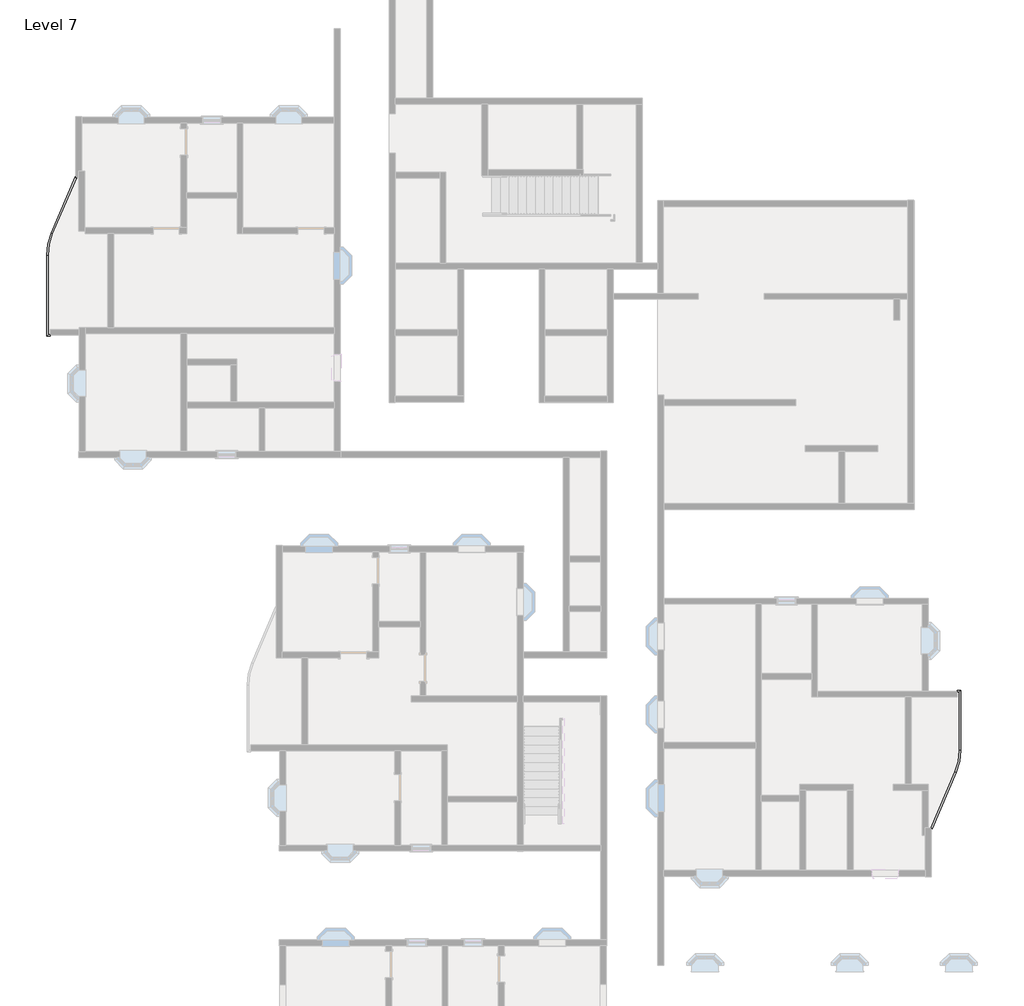
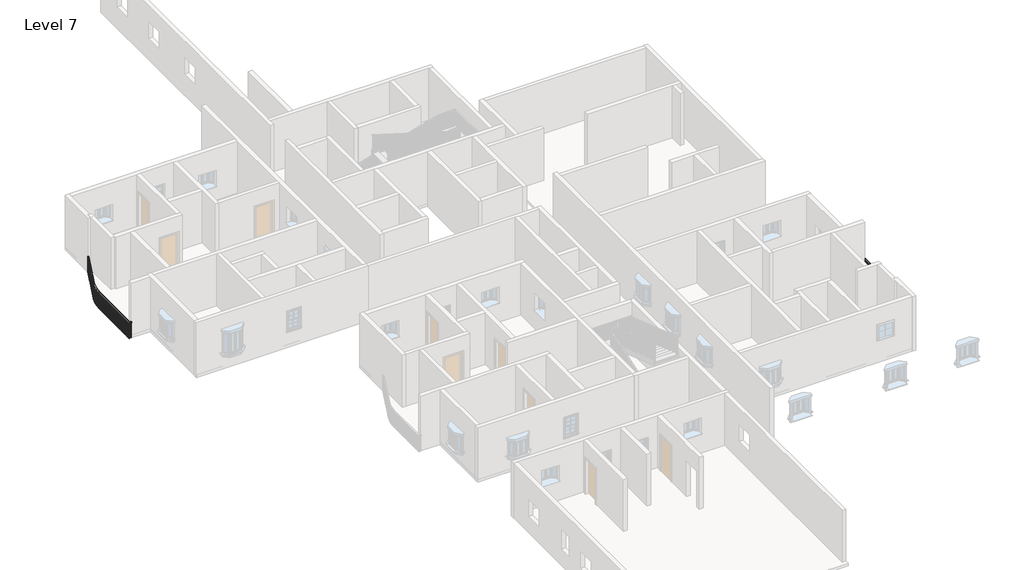
# One storey, part 9 of 14: 2 railings.
"""IFC4 building model written with IfcOpenShell, lengths in millimetres."""

from ifc_helpers import new_model, si_unit, frame, origin, place, context, project, spatial, polyline, circle_curve, outline, extrude, element, save
from ifc_brep_helpers import plane_surface, cylinder_surface, revolved_surface, advanced_brep

model = new_model("IFC4")

# Units and contexts
model_context = context("Model", 3, world=origin())
ifc_project = project(units=[si_unit("LENGTHUNIT", "METRE", prefix="MILLI")], contexts=[model_context])

# Site, building, storey
site = spatial("IfcSite", under=ifc_project)
building = spatial("IfcBuilding", under=site)
storey = spatial("IfcBuildingStorey", under=building, Name="Level 7", Elevation=18288.0)

# Railings
placement = place(None, origin())
element("IfcRailing", 1, ObjectType="Handrail - Rectangular", at=placement, inside=storey, context=model_context, shape_type="SolidModel", body=[
    advanced_brep(
    [(-19327.739878, 12446.0257339, 19202.4), (-19327.739878, 12446.0257339, 19151.6), (-19374.4383922, 12466.022953, 19151.6), (-19374.4383922, 12466.022953, 19202.4), (-20162.483418, 10496.6905323, 19202.4), (-20162.483418, 10496.6905323, 19151.6), (-20209.1819322, 10516.6877514, 19151.6), (-20209.1819322, 10516.6877514, 19202.4), (-20316.2891351, 9746.7948172, 19151.6), (-20316.2891351, 9746.7948172, 19202.4), (-20367.0891351, 9746.7948172, 19151.6), (-20367.0891351, 9746.7948172, 19202.4), (-20316.2891351, 7005.2583494, 19202.4), (-20316.2891351, 7005.2583494, 19151.6), (-20367.0891351, 6954.4583494, 19151.6), (-20367.0891351, 6954.4583494, 19202.4), (-20240.0891351, 7005.2583494, 19202.4), (-20240.0891351, 6954.4583494, 19202.4), (-20240.0891351, 6954.4583494, 19151.6), (-20240.0891351, 7005.2583494, 19151.6)],
    [
        (0, 1),
        (1, 2),
        (2, 3),
        (3, 0),
        (0, 4),
        (4, 5),
        (5, 1),
        (5, 6),
        (6, 2),
        (6, 7),
        (7, 3),
        (7, 4),
        (8, 5, circle_curve(frame((-18411.2891351, 9746.7948172, 19151.6), z_axis=(0.0, 0.0, -1.0), x_axis=(-0.919262090762392, 0.3936460446735823, 0.0)), 1905.0)),
        (4, 9, circle_curve(frame((-18411.2891351, 9746.7948172, 19202.4), z_axis=(0.0, 0.0, 1.0), x_axis=(-0.919262090762392, 0.3936460446735823, 0.0)), 1905.0)),
        (9, 8),
        (10, 6, circle_curve(frame((-18411.2891351, 9746.7948172, 19151.6), z_axis=(0.0, 0.0, -1.0), x_axis=(-0.919262090762392, 0.3936460446735823, 0.0)), 1955.8)),
        (8, 10),
        (11, 7, circle_curve(frame((-18411.2891351, 9746.7948172, 19202.4), z_axis=(0.0, 0.0, -1.0), x_axis=(-0.919262090762392, 0.3936460446735823, 0.0)), 1955.8)),
        (10, 11),
        (11, 9),
        (9, 12),
        (12, 13),
        (13, 8),
        (13, 14),
        (14, 10),
        (14, 15),
        (15, 11),
        (15, 12),
        (16, 17),
        (17, 18),
        (18, 19),
        (19, 16),
        (12, 16),
        (19, 13),
        (18, 14),
        (17, 15),
    ],
    [
        plane_surface(frame((-19351.0891351, 12456.0243434, 19202.4), z_axis=(0.3936460446735829, 0.9192620907623917, 0.0), x_axis=(0.9192620907623917, -0.3936460446735829, 0.0))),
        plane_surface(frame((-19327.739878, 12446.0257339, 19202.4), z_axis=(0.9192620907623915, -0.3936460446735834, 0.0), x_axis=(-0.3936460446735834, -0.9192620907623915, 0.0))),
        plane_surface(frame((-19327.739878, 12446.0257339, 19151.6), z_axis=(0.0, 0.0, -1.0000000000000002), x_axis=(-0.3936460446735834, -0.9192620907623915, 0.0))),
        plane_surface(frame((-19374.4383922, 12466.022953, 19151.6), z_axis=(-0.9192620907623916, 0.393646044673583, 0.0), x_axis=(-0.393646044673583, -0.9192620907623916, 0.0))),
        plane_surface(frame((-19374.4383922, 12466.022953, 19202.4), z_axis=(0.0, 0.0, 1.0), x_axis=(-0.393646044673583, -0.9192620907623916, 0.0))),
        revolved_surface(polyline([(-20162.483418002357, 10496.690532303173, 19202.4), (-20162.483418002357, 10496.690532303173, 19151.6)]), (-18411.2891351, 9746.7948172, 19202.4), (0.0, 0.0, 1.0)),
        plane_surface(frame((-18411.2891351, 9746.7948172, 19151.6), z_axis=(0.0, 0.0, -1.0), x_axis=(-0.919262090762392, 0.3936460446735823, 0.0))),
        cylinder_surface(frame((-18411.2891351, 9746.7948172, 19202.4), z_axis=(0.0, 0.0, 1.0), x_axis=(-0.919262090762392, 0.3936460446735823, 0.0)), 1955.8),
        plane_surface(frame((-18411.2891351, 9746.7948172, 19202.4), z_axis=(0.0, 0.0, 1.0), x_axis=(-0.919262090762392, 0.3936460446735823, 0.0))),
        plane_surface(frame((-20316.2891351, 9746.7948172, 19202.4), z_axis=(1.0, 0.0, 0.0), x_axis=(0.0, -1.0, 0.0))),
        plane_surface(frame((-20316.2891351, 9746.7948172, 19151.6), z_axis=(0.0, 0.0, -1.0), x_axis=(0.0, -1.0, 0.0))),
        plane_surface(frame((-20367.0891351, 9746.7948172, 19151.6), z_axis=(-1.0, 0.0, 0.0), x_axis=(0.0, -1.0, 0.0))),
        plane_surface(frame((-20367.0891351, 9746.7948172, 19202.4), z_axis=(0.0, 0.0, 1.0), x_axis=(0.0, -1.0, 0.0))),
        plane_surface(frame((-20240.0891351, 6979.8583494, 19202.4), z_axis=(1.0, 0.0, 0.0), x_axis=(0.0, 1.0, 0.0))),
        plane_surface(frame((-20316.2891351, 7005.2583494, 19202.4), z_axis=(0.0, 1.0, 0.0), x_axis=(1.0, 0.0, 0.0))),
        plane_surface(frame((-20316.2891351, 7005.2583494, 19151.6), z_axis=(0.0, 0.0, -1.0), x_axis=(1.0, 0.0, 0.0))),
        plane_surface(frame((-20367.0891351, 6954.4583494, 19151.6), z_axis=(0.0, -1.0, 0.0), x_axis=(1.0, 0.0, 0.0))),
        plane_surface(frame((-20367.0891351, 6954.4583494, 19202.4), z_axis=(0.0, 0.0, 1.0), x_axis=(1.0, 0.0, 0.0))),
    ],
    [
        (0, [[1, 2, 3, 4]]),
        (1, [[-1, 5, 6, 7]]),
        (2, [[-2, -7, 8, 9]]),
        (3, [[-3, -9, 10, 11]]),
        (4, [[-4, -11, 12, -5]]),
        (5, [[13, -6, 14, 15]]),
        (6, [[16, -8, -13, 17]]),
        (7, [[18, -10, -16, 19]]),
        (8, [[-14, -12, -18, 20]]),
        (9, [[-15, 21, 22, 23]]),
        (10, [[-17, -23, 24, 25]]),
        (11, [[-19, -25, 26, 27]]),
        (12, [[-20, -27, 28, -21]]),
        (13, [[29, 30, 31, 32]]),
        (14, [[-22, 33, -32, 34]]),
        (15, [[-24, -34, -31, 35]]),
        (16, [[-26, -35, -30, 36]]),
        (17, [[-28, -36, -29, -33]]),
    ],
),
    extrude(outline(polyline([(-20351.2141351, 7013.1198172), (-20332.1641351, 7013.1198172), (-20332.1641351, 6994.0698172), (-20351.2141351, 6994.0698172), (-20351.2141351, 7013.1198172)])), frame((0.0, 0.0, 18288.0), z_axis=(0.0, 0.0, 1.0), x_axis=(1.0, 0.0, 0.0)), (0.0, 0.0, 1.0), 863.6),
    extrude(outline(polyline([(-20351.2141351, 7114.7198172), (-20332.1641351, 7114.7198172), (-20332.1641351, 7095.6698172), (-20351.2141351, 7095.6698172), (-20351.2141351, 7114.7198172)])), frame((0.0, 0.0, 18288.0), z_axis=(0.0, 0.0, 1.0), x_axis=(1.0, 0.0, 0.0)), (0.0, 0.0, 1.0), 863.6),
    extrude(outline(polyline([(-20351.2141351, 7216.3198172), (-20332.1641351, 7216.3198172), (-20332.1641351, 7197.2698172), (-20351.2141351, 7197.2698172), (-20351.2141351, 7216.3198172)])), frame((0.0, 0.0, 18288.0), z_axis=(0.0, 0.0, 1.0), x_axis=(1.0, 0.0, 0.0)), (0.0, 0.0, 1.0), 863.6),
    extrude(outline(polyline([(-20351.2141351, 7317.9198172), (-20332.1641351, 7317.9198172), (-20332.1641351, 7298.8698172), (-20351.2141351, 7298.8698172), (-20351.2141351, 7317.9198172)])), frame((0.0, 0.0, 18288.0), z_axis=(0.0, 0.0, 1.0), x_axis=(1.0, 0.0, 0.0)), (0.0, 0.0, 1.0), 863.6),
    extrude(outline(polyline([(-20351.2141351, 7419.5198172), (-20332.1641351, 7419.5198172), (-20332.1641351, 7400.4698172), (-20351.2141351, 7400.4698172), (-20351.2141351, 7419.5198172)])), frame((0.0, 0.0, 18288.0), z_axis=(0.0, 0.0, 1.0), x_axis=(1.0, 0.0, 0.0)), (0.0, 0.0, 1.0), 863.6),
    extrude(outline(polyline([(-20351.2141351, 7521.1198172), (-20332.1641351, 7521.1198172), (-20332.1641351, 7502.0698172), (-20351.2141351, 7502.0698172), (-20351.2141351, 7521.1198172)])), frame((0.0, 0.0, 18288.0), z_axis=(0.0, 0.0, 1.0), x_axis=(1.0, 0.0, 0.0)), (0.0, 0.0, 1.0), 863.6),
    extrude(outline(polyline([(-20351.2141351, 7622.7198172), (-20332.1641351, 7622.7198172), (-20332.1641351, 7603.6698172), (-20351.2141351, 7603.6698172), (-20351.2141351, 7622.7198172)])), frame((0.0, 0.0, 18288.0), z_axis=(0.0, 0.0, 1.0), x_axis=(1.0, 0.0, 0.0)), (0.0, 0.0, 1.0), 863.6),
    extrude(outline(polyline([(-20351.2141351, 7724.3198172), (-20332.1641351, 7724.3198172), (-20332.1641351, 7705.2698172), (-20351.2141351, 7705.2698172), (-20351.2141351, 7724.3198172)])), frame((0.0, 0.0, 18288.0), z_axis=(0.0, 0.0, 1.0), x_axis=(1.0, 0.0, 0.0)), (0.0, 0.0, 1.0), 863.6),
    extrude(outline(polyline([(-20351.2141351, 7825.9198172), (-20332.1641351, 7825.9198172), (-20332.1641351, 7806.8698172), (-20351.2141351, 7806.8698172), (-20351.2141351, 7825.9198172)])), frame((0.0, 0.0, 18288.0), z_axis=(0.0, 0.0, 1.0), x_axis=(1.0, 0.0, 0.0)), (0.0, 0.0, 1.0), 863.6),
    extrude(outline(polyline([(-20351.2141351, 7927.5198172), (-20332.1641351, 7927.5198172), (-20332.1641351, 7908.4698172), (-20351.2141351, 7908.4698172), (-20351.2141351, 7927.5198172)])), frame((0.0, 0.0, 18288.0), z_axis=(0.0, 0.0, 1.0), x_axis=(1.0, 0.0, 0.0)), (0.0, 0.0, 1.0), 863.6),
    extrude(outline(polyline([(-20351.2141351, 8029.1198172), (-20332.1641351, 8029.1198172), (-20332.1641351, 8010.0698172), (-20351.2141351, 8010.0698172), (-20351.2141351, 8029.1198172)])), frame((0.0, 0.0, 18288.0), z_axis=(0.0, 0.0, 1.0), x_axis=(1.0, 0.0, 0.0)), (0.0, 0.0, 1.0), 863.6),
    extrude(outline(polyline([(-20351.2141351, 8130.7198172), (-20332.1641351, 8130.7198172), (-20332.1641351, 8111.6698172), (-20351.2141351, 8111.6698172), (-20351.2141351, 8130.7198172)])), frame((0.0, 0.0, 18288.0), z_axis=(0.0, 0.0, 1.0), x_axis=(1.0, 0.0, 0.0)), (0.0, 0.0, 1.0), 863.6),
    extrude(outline(polyline([(-20351.2141351, 8232.3198172), (-20332.1641351, 8232.3198172), (-20332.1641351, 8213.2698172), (-20351.2141351, 8213.2698172), (-20351.2141351, 8232.3198172)])), frame((0.0, 0.0, 18288.0), z_axis=(0.0, 0.0, 1.0), x_axis=(1.0, 0.0, 0.0)), (0.0, 0.0, 1.0), 863.6),
    extrude(outline(polyline([(-20351.2141351, 8333.9198172), (-20332.1641351, 8333.9198172), (-20332.1641351, 8314.8698172), (-20351.2141351, 8314.8698172), (-20351.2141351, 8333.9198172)])), frame((0.0, 0.0, 18288.0), z_axis=(0.0, 0.0, 1.0), x_axis=(1.0, 0.0, 0.0)), (0.0, 0.0, 1.0), 863.6),
    extrude(outline(polyline([(-20351.2141351, 8435.5198172), (-20332.1641351, 8435.5198172), (-20332.1641351, 8416.4698172), (-20351.2141351, 8416.4698172), (-20351.2141351, 8435.5198172)])), frame((0.0, 0.0, 18288.0), z_axis=(0.0, 0.0, 1.0), x_axis=(1.0, 0.0, 0.0)), (0.0, 0.0, 1.0), 863.6),
    extrude(outline(polyline([(-20351.2141351, 8537.1198172), (-20332.1641351, 8537.1198172), (-20332.1641351, 8518.0698172), (-20351.2141351, 8518.0698172), (-20351.2141351, 8537.1198172)])), frame((0.0, 0.0, 18288.0), z_axis=(0.0, 0.0, 1.0), x_axis=(1.0, 0.0, 0.0)), (0.0, 0.0, 1.0), 863.6),
    extrude(outline(polyline([(-20351.2141351, 8638.7198172), (-20332.1641351, 8638.7198172), (-20332.1641351, 8619.6698172), (-20351.2141351, 8619.6698172), (-20351.2141351, 8638.7198172)])), frame((0.0, 0.0, 18288.0), z_axis=(0.0, 0.0, 1.0), x_axis=(1.0, 0.0, 0.0)), (0.0, 0.0, 1.0), 863.6),
    extrude(outline(polyline([(-20351.2141351, 8740.3198172), (-20332.1641351, 8740.3198172), (-20332.1641351, 8721.2698172), (-20351.2141351, 8721.2698172), (-20351.2141351, 8740.3198172)])), frame((0.0, 0.0, 18288.0), z_axis=(0.0, 0.0, 1.0), x_axis=(1.0, 0.0, 0.0)), (0.0, 0.0, 1.0), 863.6),
    extrude(outline(polyline([(-20351.2141351, 8841.9198172), (-20332.1641351, 8841.9198172), (-20332.1641351, 8822.8698172), (-20351.2141351, 8822.8698172), (-20351.2141351, 8841.9198172)])), frame((0.0, 0.0, 18288.0), z_axis=(0.0, 0.0, 1.0), x_axis=(1.0, 0.0, 0.0)), (0.0, 0.0, 1.0), 863.6),
    extrude(outline(polyline([(-20351.2141351, 8943.5198172), (-20332.1641351, 8943.5198172), (-20332.1641351, 8924.4698172), (-20351.2141351, 8924.4698172), (-20351.2141351, 8943.5198172)])), frame((0.0, 0.0, 18288.0), z_axis=(0.0, 0.0, 1.0), x_axis=(1.0, 0.0, 0.0)), (0.0, 0.0, 1.0), 863.6),
    extrude(outline(polyline([(-20351.2141351, 9045.1198172), (-20332.1641351, 9045.1198172), (-20332.1641351, 9026.0698172), (-20351.2141351, 9026.0698172), (-20351.2141351, 9045.1198172)])), frame((0.0, 0.0, 18288.0), z_axis=(0.0, 0.0, 1.0), x_axis=(1.0, 0.0, 0.0)), (0.0, 0.0, 1.0), 863.6),
    extrude(outline(polyline([(-20351.2141351, 9146.7198172), (-20332.1641351, 9146.7198172), (-20332.1641351, 9127.6698172), (-20351.2141351, 9127.6698172), (-20351.2141351, 9146.7198172)])), frame((0.0, 0.0, 18288.0), z_axis=(0.0, 0.0, 1.0), x_axis=(1.0, 0.0, 0.0)), (0.0, 0.0, 1.0), 863.6),
    extrude(outline(polyline([(-20351.2141351, 9248.3198172), (-20332.1641351, 9248.3198172), (-20332.1641351, 9229.2698172), (-20351.2141351, 9229.2698172), (-20351.2141351, 9248.3198172)])), frame((0.0, 0.0, 18288.0), z_axis=(0.0, 0.0, 1.0), x_axis=(1.0, 0.0, 0.0)), (0.0, 0.0, 1.0), 863.6),
    extrude(outline(polyline([(-20351.2141351, 9349.9198172), (-20332.1641351, 9349.9198172), (-20332.1641351, 9330.8698172), (-20351.2141351, 9330.8698172), (-20351.2141351, 9349.9198172)])), frame((0.0, 0.0, 18288.0), z_axis=(0.0, 0.0, 1.0), x_axis=(1.0, 0.0, 0.0)), (0.0, 0.0, 1.0), 863.6),
    extrude(outline(polyline([(-20351.2141351, 9451.5198172), (-20332.1641351, 9451.5198172), (-20332.1641351, 9432.4698172), (-20351.2141351, 9432.4698172), (-20351.2141351, 9451.5198172)])), frame((0.0, 0.0, 18288.0), z_axis=(0.0, 0.0, 1.0), x_axis=(1.0, 0.0, 0.0)), (0.0, 0.0, 1.0), 863.6),
    extrude(outline(polyline([(-20351.2141351, 9553.1198172), (-20332.1641351, 9553.1198172), (-20332.1641351, 9534.0698172), (-20351.2141351, 9534.0698172), (-20351.2141351, 9553.1198172)])), frame((0.0, 0.0, 18288.0), z_axis=(0.0, 0.0, 1.0), x_axis=(1.0, 0.0, 0.0)), (0.0, 0.0, 1.0), 863.6),
    extrude(outline(polyline([(-20351.2141351, 9654.7198172), (-20332.1641351, 9654.7198172), (-20332.1641351, 9635.6698172), (-20351.2141351, 9635.6698172), (-20351.2141351, 9654.7198172)])), frame((0.0, 0.0, 18288.0), z_axis=(0.0, 0.0, 1.0), x_axis=(1.0, 0.0, 0.0)), (0.0, 0.0, 1.0), 863.6),
    extrude(outline(polyline([(-20349.6005818, 9826.4720848), (-20330.5630441, 9825.7831307), (-20331.2519982, 9806.745593), (-20350.289536, 9807.4345471), (-20349.6005818, 9826.4720848)])), frame((0.0, 0.0, 18288.0), z_axis=(0.0, 0.0, 1.0), x_axis=(1.0, 0.0, 0.0)), (0.0, 0.0, 1.0), 863.6),
    extrude(outline(polyline([(-20342.724955, 9928.3310534), (-20323.750023, 9926.6415402), (-20325.4395363, 9907.6666081), (-20344.4144683, 9909.3561214), (-20342.724955, 9928.3310534)])), frame((0.0, 0.0, 18288.0), z_axis=(0.0, 0.0, 1.0), x_axis=(1.0, 0.0, 0.0)), (0.0, 0.0, 1.0), 863.6),
    extrude(outline(polyline([(-20330.5003254, 10029.6872677), (-20311.6405491, 10027.0018743), (-20314.3259425, 10008.142098), (-20333.1857188, 10010.8274914), (-20330.5003254, 10029.6872677)])), frame((0.0, 0.0, 18288.0), z_axis=(0.0, 0.0, 1.0), x_axis=(1.0, 0.0, 0.0)), (0.0, 0.0, 1.0), 863.6),
    extrude(outline(polyline([(-20312.9605484, 10130.2600272), (-20294.2681589, 10126.5861907), (-20297.9419954, 10107.8938012), (-20316.6343849, 10111.5676377), (-20312.9605484, 10130.2600272)])), frame((0.0, 0.0, 18288.0), z_axis=(0.0, 0.0, 1.0), x_axis=(1.0, 0.0, 0.0)), (0.0, 0.0, 1.0), 863.6),
    extrude(outline(polyline([(-20290.1541995, 10229.7708014), (-20271.6809643, 10225.1186963), (-20276.3330693, 10206.6454611), (-20294.8063045, 10211.2975662), (-20290.1541995, 10229.7708014)])), frame((0.0, 0.0, 18288.0), z_axis=(0.0, 0.0, 1.0), x_axis=(1.0, 0.0, 0.0)), (0.0, 0.0, 1.0), 863.6),
    extrude(outline(polyline([(-20262.1444395, 10327.9440008), (-20243.9415192, 10322.3265109), (-20249.5590091, 10304.1235906), (-20267.7619294, 10309.7410805), (-20262.1444395, 10327.9440008)])), frame((0.0, 0.0, 18288.0), z_axis=(0.0, 0.0, 1.0), x_axis=(1.0, 0.0, 0.0)), (0.0, 0.0, 1.0), 863.6),
    extrude(outline(polyline([(-20229.0088399, 10424.5077402), (-20211.1266465, 10417.9404228), (-20217.693964, 10400.0582293), (-20235.5761574, 10406.6255468), (-20229.0088399, 10424.5077402)])), frame((0.0, 0.0, 18288.0), z_axis=(0.0, 0.0, 1.0), x_axis=(1.0, 0.0, 0.0)), (0.0, 0.0, 1.0), 863.6),
    extrude(outline(polyline([(-20155.9843907, 10600.589225), (-20138.4724479, 10593.0902678), (-20145.9714051, 10575.578325), (-20163.4833479, 10583.0772822), (-20155.9843907, 10600.589225)])), frame((0.0, 0.0, 18288.0), z_axis=(0.0, 0.0, 1.0), x_axis=(1.0, 0.0, 0.0)), (0.0, 0.0, 1.0), 863.6),
    extrude(outline(polyline([(-20115.9899526, 10693.9862534), (-20098.4780098, 10686.4872963), (-20105.9769669, 10668.9753534), (-20123.4889098, 10676.4743106), (-20115.9899526, 10693.9862534)])), frame((0.0, 0.0, 18288.0), z_axis=(0.0, 0.0, 1.0), x_axis=(1.0, 0.0, 0.0)), (0.0, 0.0, 1.0), 863.6),
    extrude(outline(polyline([(-20075.9955145, 10787.3832818), (-20058.4835716, 10779.8843247), (-20065.9825288, 10762.3723818), (-20083.4944716, 10769.871339), (-20075.9955145, 10787.3832818)])), frame((0.0, 0.0, 18288.0), z_axis=(0.0, 0.0, 1.0), x_axis=(1.0, 0.0, 0.0)), (0.0, 0.0, 1.0), 863.6),
    extrude(outline(polyline([(-20036.0010763, 10880.7803103), (-20018.4891335, 10873.2813531), (-20025.9880906, 10855.7694103), (-20043.5000335, 10863.2683674), (-20036.0010763, 10880.7803103)])), frame((0.0, 0.0, 18288.0), z_axis=(0.0, 0.0, 1.0), x_axis=(1.0, 0.0, 0.0)), (0.0, 0.0, 1.0), 863.6),
    extrude(outline(polyline([(-19996.0066382, 10974.1773387), (-19978.4946954, 10966.6783815), (-19985.9936525, 10949.1664387), (-20003.5055953, 10956.6653958), (-19996.0066382, 10974.1773387)])), frame((0.0, 0.0, 18288.0), z_axis=(0.0, 0.0, 1.0), x_axis=(1.0, 0.0, 0.0)), (0.0, 0.0, 1.0), 863.6),
    extrude(outline(polyline([(-19956.0122, 11067.5743671), (-19938.5002572, 11060.0754099), (-19945.9992144, 11042.5634671), (-19963.5111572, 11050.0624243), (-19956.0122, 11067.5743671)])), frame((0.0, 0.0, 18288.0), z_axis=(0.0, 0.0, 1.0), x_axis=(1.0, 0.0, 0.0)), (0.0, 0.0, 1.0), 863.6),
    extrude(outline(polyline([(-19916.0177619, 11160.9713955), (-19898.5058191, 11153.4724384), (-19906.0047762, 11135.9604955), (-19923.5167191, 11143.4594527), (-19916.0177619, 11160.9713955)])), frame((0.0, 0.0, 18288.0), z_axis=(0.0, 0.0, 1.0), x_axis=(1.0, 0.0, 0.0)), (0.0, 0.0, 1.0), 863.6),
    extrude(outline(polyline([(-19876.0233238, 11254.3684239), (-19858.5113809, 11246.8694668), (-19866.0103381, 11229.357524), (-19883.5222809, 11236.8564811), (-19876.0233238, 11254.3684239)])), frame((0.0, 0.0, 18288.0), z_axis=(0.0, 0.0, 1.0), x_axis=(1.0, 0.0, 0.0)), (0.0, 0.0, 1.0), 863.6),
    extrude(outline(polyline([(-19836.0288856, 11347.7654524), (-19818.5169428, 11340.2664952), (-19826.0159, 11322.7545524), (-19843.5278428, 11330.2535095), (-19836.0288856, 11347.7654524)])), frame((0.0, 0.0, 18288.0), z_axis=(0.0, 0.0, 1.0), x_axis=(1.0, 0.0, 0.0)), (0.0, 0.0, 1.0), 863.6),
    extrude(outline(polyline([(-19796.0344475, 11441.1624808), (-19778.5225047, 11433.6635236), (-19786.0214618, 11416.1515808), (-19803.5334046, 11423.650538), (-19796.0344475, 11441.1624808)])), frame((0.0, 0.0, 18288.0), z_axis=(0.0, 0.0, 1.0), x_axis=(1.0, 0.0, 0.0)), (0.0, 0.0, 1.0), 863.6),
    extrude(outline(polyline([(-19756.0400094, 11534.5595092), (-19738.5280665, 11527.060552), (-19746.0270237, 11509.5486092), (-19763.5389665, 11517.0475664), (-19756.0400094, 11534.5595092)])), frame((0.0, 0.0, 18288.0), z_axis=(0.0, 0.0, 1.0), x_axis=(1.0, 0.0, 0.0)), (0.0, 0.0, 1.0), 863.6),
    extrude(outline(polyline([(-19716.0455712, 11627.9565376), (-19698.5336284, 11620.4575805), (-19706.0325855, 11602.9456376), (-19723.5445284, 11610.4445948), (-19716.0455712, 11627.9565376)])), frame((0.0, 0.0, 18288.0), z_axis=(0.0, 0.0, 1.0), x_axis=(1.0, 0.0, 0.0)), (0.0, 0.0, 1.0), 863.6),
    extrude(outline(polyline([(-19676.0511331, 11721.353566), (-19658.5391902, 11713.8546089), (-19666.0381474, 11696.3426661), (-19683.5500902, 11703.8416232), (-19676.0511331, 11721.353566)])), frame((0.0, 0.0, 18288.0), z_axis=(0.0, 0.0, 1.0), x_axis=(1.0, 0.0, 0.0)), (0.0, 0.0, 1.0), 863.6),
    extrude(outline(polyline([(-19636.0566949, 11814.7505945), (-19618.5447521, 11807.2516373), (-19626.0437093, 11789.7396945), (-19643.5556521, 11797.2386516), (-19636.0566949, 11814.7505945)])), frame((0.0, 0.0, 18288.0), z_axis=(0.0, 0.0, 1.0), x_axis=(1.0, 0.0, 0.0)), (0.0, 0.0, 1.0), 863.6),
    extrude(outline(polyline([(-19596.0622568, 11908.1476229), (-19578.550314, 11900.6486657), (-19586.0492711, 11883.1367229), (-19603.561214, 11890.6356801), (-19596.0622568, 11908.1476229)])), frame((0.0, 0.0, 18288.0), z_axis=(0.0, 0.0, 1.0), x_axis=(1.0, 0.0, 0.0)), (0.0, 0.0, 1.0), 863.6),
    extrude(outline(polyline([(-19556.0678187, 12001.5446513), (-19538.5558758, 11994.0456942), (-19546.054833, 11976.5337513), (-19563.5667758, 11984.0327085), (-19556.0678187, 12001.5446513)])), frame((0.0, 0.0, 18288.0), z_axis=(0.0, 0.0, 1.0), x_axis=(1.0, 0.0, 0.0)), (0.0, 0.0, 1.0), 863.6),
    extrude(outline(polyline([(-19516.0733805, 12094.9416797), (-19498.5614377, 12087.4427226), (-19506.0603948, 12069.9307797), (-19523.5723377, 12077.4297369), (-19516.0733805, 12094.9416797)])), frame((0.0, 0.0, 18288.0), z_axis=(0.0, 0.0, 1.0), x_axis=(1.0, 0.0, 0.0)), (0.0, 0.0, 1.0), 863.6),
    extrude(outline(polyline([(-19476.0789424, 12188.3387082), (-19458.5669996, 12180.839751), (-19466.0659567, 12163.3278082), (-19483.5778995, 12170.8267653), (-19476.0789424, 12188.3387082)])), frame((0.0, 0.0, 18288.0), z_axis=(0.0, 0.0, 1.0), x_axis=(1.0, 0.0, 0.0)), (0.0, 0.0, 1.0), 863.6),
    extrude(outline(polyline([(-19436.0845042, 12281.7357366), (-19418.5725614, 12274.2367794), (-19426.0715186, 12256.7248366), (-19443.5834614, 12264.2237937), (-19436.0845042, 12281.7357366)])), frame((0.0, 0.0, 18288.0), z_axis=(0.0, 0.0, 1.0), x_axis=(1.0, 0.0, 0.0)), (0.0, 0.0, 1.0), 863.6),
    extrude(outline(polyline([(-19396.0900661, 12375.132765), (-19378.5781233, 12367.6338078), (-19386.0770804, 12350.121865), (-19403.5890233, 12357.6208222), (-19396.0900661, 12375.132765)])), frame((0.0, 0.0, 18288.0), z_axis=(0.0, 0.0, 1.0), x_axis=(1.0, 0.0, 0.0)), (0.0, 0.0, 1.0), 863.6),
    extrude(outline(polyline([(-20351.2141351, 6989.3833494), (-20332.1641351, 6989.3833494), (-20332.1641351, 6970.3333494), (-20351.2141351, 6970.3333494), (-20351.2141351, 6989.3833494)])), frame((0.0, 0.0, 18288.0), z_axis=(0.0, 0.0, 1.0), x_axis=(1.0, 0.0, 0.0)), (0.0, 0.0, 1.0), 863.6),
    extrude(outline(polyline([(-20351.2141351, 9756.3198172), (-20332.1641351, 9756.3198172), (-20332.1641351, 9737.2698172), (-20351.2141351, 9737.2698172), (-20351.2141351, 9756.3198172)])), frame((0.0, 0.0, 18288.0), z_axis=(0.0, 0.0, 1.0), x_axis=(1.0, 0.0, 0.0)), (0.0, 0.0, 1.0), 863.6),
    extrude(outline(polyline([(-20190.839168, 10519.1945919), (-20173.3272251, 10511.6956347), (-20180.8261823, 10494.1836919), (-20198.3381251, 10501.682649), (-20190.839168, 10519.1945919)])), frame((0.0, 0.0, 18288.0), z_axis=(0.0, 0.0, 1.0), x_axis=(1.0, 0.0, 0.0)), (0.0, 0.0, 1.0), 863.6),
    extrude(outline(polyline([(-20259.1391351, 6970.3333494), (-20259.1391351, 6989.3833494), (-20240.0891351, 6989.3833494), (-20240.0891351, 6970.3333494), (-20259.1391351, 6970.3333494)])), frame((0.0, 0.0, 18288.0), z_axis=(0.0, 0.0, 1.0), x_axis=(1.0, 0.0, 0.0)), (0.0, 0.0, 1.0), 863.6),
    extrude(outline(polyline([(-19359.8451065, 12459.773822), (-19342.3331637, 12452.2748648), (-19349.8321209, 12434.762922), (-19367.3440637, 12442.2618792), (-19359.8451065, 12459.773822)])), frame((0.0, 0.0, 18288.0), z_axis=(0.0, 0.0, 1.0), x_axis=(1.0, 0.0, 0.0)), (0.0, 0.0, 1.0), 863.6),
])
element("IfcRailing", 2, ObjectType="Handrail - Rectangular", at=placement, inside=storey, context=model_context, shape_type="SolidModel", body=[
    advanced_brep(
    [(10250.7887952, -10096.81198, 19202.4), (10250.7887952, -10096.81198, 19151.6), (10297.4873094, -10116.8091991, 19151.6), (10297.4873094, -10116.8091991, 19202.4), (11085.5323352, -8147.4767784, 19202.4), (11085.5323352, -8147.4767784, 19151.6), (11132.2308494, -8167.4739975, 19151.6), (11132.2308494, -8167.4739975, 19202.4), (11239.3380523, -7397.5810633, 19151.6), (11239.3380523, -7397.5810633, 19202.4), (11290.1380523, -7397.5810633, 19151.6), (11290.1380523, -7397.5810633, 19202.4), (11239.3380523, -5378.0542694, 19202.4), (11239.3380523, -5378.0542694, 19151.6), (11290.1380523, -5327.2542694, 19151.6), (11290.1380523, -5327.2542694, 19202.4), (11163.1380523, -5378.0542694, 19202.4), (11163.1380523, -5327.2542694, 19202.4), (11163.1380523, -5327.2542694, 19151.6), (11163.1380523, -5378.0542694, 19151.6)],
    [
        (0, 1),
        (1, 2),
        (2, 3),
        (3, 0),
        (0, 4),
        (4, 5),
        (5, 1),
        (5, 6),
        (6, 2),
        (6, 7),
        (7, 3),
        (7, 4),
        (8, 5, circle_curve(frame((9334.3380523, -7397.5810633, 19151.6), z_axis=(0.0, 0.0, -1.0), x_axis=(0.9192620907624003, -0.3936460446735628, 0.0)), 1905.0)),
        (4, 9, circle_curve(frame((9334.3380523, -7397.5810633, 19202.4), z_axis=(0.0, 0.0, 1.0), x_axis=(0.9192620907624003, -0.3936460446735628, 0.0)), 1905.0)),
        (9, 8),
        (10, 6, circle_curve(frame((9334.3380523, -7397.5810633, 19151.6), z_axis=(0.0, 0.0, -1.0), x_axis=(0.9192620907624003, -0.3936460446735628, 0.0)), 1955.8)),
        (8, 10),
        (11, 7, circle_curve(frame((9334.3380523, -7397.5810633, 19202.4), z_axis=(0.0, 0.0, -1.0), x_axis=(0.9192620907624003, -0.3936460446735628, 0.0)), 1955.8)),
        (10, 11),
        (11, 9),
        (9, 12),
        (12, 13),
        (13, 8),
        (13, 14),
        (14, 10),
        (14, 15),
        (15, 11),
        (15, 12),
        (16, 17),
        (17, 18),
        (18, 19),
        (19, 16),
        (12, 16),
        (19, 13),
        (18, 14),
        (17, 15),
    ],
    [
        plane_surface(frame((10274.1380523, -10106.8105895, 19202.4), z_axis=(-0.3936460446735629, -0.9192620907624003, 0.0), x_axis=(0.9192620907624003, -0.3936460446735629, 0.0))),
        plane_surface(frame((10250.7887952, -10096.81198, 19202.4), z_axis=(-0.9192620907624005, 0.39364604467356235, 0.0), x_axis=(0.39364604467356235, 0.9192620907624005, 0.0))),
        plane_surface(frame((10250.7887952, -10096.81198, 19151.6), z_axis=(0.0, 0.0, -1.0), x_axis=(0.39364604467356235, 0.9192620907624005, 0.0))),
        plane_surface(frame((10297.4873094, -10116.8091991, 19151.6), z_axis=(0.9192620907624003, -0.3936460446735627, 0.0), x_axis=(0.3936460446735627, 0.9192620907624003, 0.0))),
        plane_surface(frame((10297.4873094, -10116.8091991, 19202.4), z_axis=(0.0, 0.0, 1.0), x_axis=(0.3936460446735627, 0.9192620907624003, 0.0))),
        revolved_surface(polyline([(11085.532335202372, -8147.476778403137, 19202.4), (11085.532335202372, -8147.476778403137, 19151.6)]), (9334.3380523, -7397.5810633, 19202.4), (0.0, 0.0, 1.0)),
        plane_surface(frame((9334.3380523, -7397.5810633, 19151.6), z_axis=(0.0, 0.0, -1.0), x_axis=(0.9192620907624003, -0.3936460446735628, 0.0))),
        cylinder_surface(frame((9334.3380523, -7397.5810633, 19202.4), z_axis=(0.0, 0.0, 1.0), x_axis=(0.9192620907624003, -0.3936460446735628, 0.0)), 1955.8),
        plane_surface(frame((9334.3380523, -7397.5810633, 19202.4), z_axis=(0.0, 0.0, 1.0), x_axis=(0.9192620907624003, -0.3936460446735628, 0.0))),
        plane_surface(frame((11239.3380523, -7397.5810633, 19202.4), z_axis=(-1.0, 0.0, 0.0), x_axis=(0.0, 1.0, 0.0))),
        plane_surface(frame((11239.3380523, -7397.5810633, 19151.6), z_axis=(0.0, 0.0, -1.0), x_axis=(0.0, 1.0, 0.0))),
        plane_surface(frame((11290.1380523, -7397.5810633, 19151.6), z_axis=(1.0, 0.0, 0.0), x_axis=(0.0, 1.0, 0.0))),
        plane_surface(frame((11290.1380523, -7397.5810633, 19202.4), z_axis=(0.0, 0.0, 1.0), x_axis=(0.0, 1.0, 0.0))),
        plane_surface(frame((11163.1380523, -5352.6542694, 19202.4), z_axis=(-1.0, 0.0, 0.0), x_axis=(0.0, -1.0, 0.0))),
        plane_surface(frame((11239.3380523, -5378.0542694, 19202.4), z_axis=(0.0, -1.0, 0.0), x_axis=(-1.0, 0.0, 0.0))),
        plane_surface(frame((11239.3380523, -5378.0542694, 19151.6), z_axis=(0.0, 0.0, -1.0), x_axis=(-1.0, 0.0, 0.0))),
        plane_surface(frame((11290.1380523, -5327.2542694, 19151.6), z_axis=(0.0, 1.0, 0.0), x_axis=(-1.0, 0.0, 0.0))),
        plane_surface(frame((11290.1380523, -5327.2542694, 19202.4), z_axis=(0.0, 0.0, 1.0), x_axis=(-1.0, 0.0, 0.0))),
    ],
    [
        (0, [[1, 2, 3, 4]]),
        (1, [[-1, 5, 6, 7]]),
        (2, [[-2, -7, 8, 9]]),
        (3, [[-3, -9, 10, 11]]),
        (4, [[-4, -11, 12, -5]]),
        (5, [[13, -6, 14, 15]]),
        (6, [[16, -8, -13, 17]]),
        (7, [[18, -10, -16, 19]]),
        (8, [[-14, -12, -18, 20]]),
        (9, [[-15, 21, 22, 23]]),
        (10, [[-17, -23, 24, 25]]),
        (11, [[-19, -25, 26, 27]]),
        (12, [[-20, -27, 28, -21]]),
        (13, [[29, 30, 31, 32]]),
        (14, [[-22, 33, -32, 34]]),
        (15, [[-24, -34, -31, 35]]),
        (16, [[-26, -35, -30, 36]]),
        (17, [[-28, -36, -29, -33]]),
    ],
),
    extrude(outline(polyline([(11274.2630523, -5375.1060633), (11255.2130523, -5375.1060633), (11255.2130523, -5356.0560633), (11274.2630523, -5356.0560633), (11274.2630523, -5375.1060633)])), frame((0.0, 0.0, 18288.0), z_axis=(0.0, 0.0, 1.0), x_axis=(1.0, 0.0, 0.0)), (0.0, 0.0, 1.0), 863.6),
    extrude(outline(polyline([(11274.2630523, -5476.7060633), (11255.2130523, -5476.7060633), (11255.2130523, -5457.6560633), (11274.2630523, -5457.6560633), (11274.2630523, -5476.7060633)])), frame((0.0, 0.0, 18288.0), z_axis=(0.0, 0.0, 1.0), x_axis=(1.0, 0.0, 0.0)), (0.0, 0.0, 1.0), 863.6),
    extrude(outline(polyline([(11274.2630523, -5578.3060633), (11255.2130523, -5578.3060633), (11255.2130523, -5559.2560633), (11274.2630523, -5559.2560633), (11274.2630523, -5578.3060633)])), frame((0.0, 0.0, 18288.0), z_axis=(0.0, 0.0, 1.0), x_axis=(1.0, 0.0, 0.0)), (0.0, 0.0, 1.0), 863.6),
    extrude(outline(polyline([(11274.2630523, -5679.9060633), (11255.2130523, -5679.9060633), (11255.2130523, -5660.8560633), (11274.2630523, -5660.8560633), (11274.2630523, -5679.9060633)])), frame((0.0, 0.0, 18288.0), z_axis=(0.0, 0.0, 1.0), x_axis=(1.0, 0.0, 0.0)), (0.0, 0.0, 1.0), 863.6),
    extrude(outline(polyline([(11274.2630523, -5781.5060633), (11255.2130523, -5781.5060633), (11255.2130523, -5762.4560633), (11274.2630523, -5762.4560633), (11274.2630523, -5781.5060633)])), frame((0.0, 0.0, 18288.0), z_axis=(0.0, 0.0, 1.0), x_axis=(1.0, 0.0, 0.0)), (0.0, 0.0, 1.0), 863.6),
    extrude(outline(polyline([(11274.2630523, -5883.1060633), (11255.2130523, -5883.1060633), (11255.2130523, -5864.0560633), (11274.2630523, -5864.0560633), (11274.2630523, -5883.1060633)])), frame((0.0, 0.0, 18288.0), z_axis=(0.0, 0.0, 1.0), x_axis=(1.0, 0.0, 0.0)), (0.0, 0.0, 1.0), 863.6),
    extrude(outline(polyline([(11274.2630523, -5984.7060633), (11255.2130523, -5984.7060633), (11255.2130523, -5965.6560633), (11274.2630523, -5965.6560633), (11274.2630523, -5984.7060633)])), frame((0.0, 0.0, 18288.0), z_axis=(0.0, 0.0, 1.0), x_axis=(1.0, 0.0, 0.0)), (0.0, 0.0, 1.0), 863.6),
    extrude(outline(polyline([(11274.2630523, -6086.3060633), (11255.2130523, -6086.3060633), (11255.2130523, -6067.2560633), (11274.2630523, -6067.2560633), (11274.2630523, -6086.3060633)])), frame((0.0, 0.0, 18288.0), z_axis=(0.0, 0.0, 1.0), x_axis=(1.0, 0.0, 0.0)), (0.0, 0.0, 1.0), 863.6),
    extrude(outline(polyline([(11274.2630523, -6187.9060633), (11255.2130523, -6187.9060633), (11255.2130523, -6168.8560633), (11274.2630523, -6168.8560633), (11274.2630523, -6187.9060633)])), frame((0.0, 0.0, 18288.0), z_axis=(0.0, 0.0, 1.0), x_axis=(1.0, 0.0, 0.0)), (0.0, 0.0, 1.0), 863.6),
    extrude(outline(polyline([(11274.2630523, -6289.5060633), (11255.2130523, -6289.5060633), (11255.2130523, -6270.4560633), (11274.2630523, -6270.4560633), (11274.2630523, -6289.5060633)])), frame((0.0, 0.0, 18288.0), z_axis=(0.0, 0.0, 1.0), x_axis=(1.0, 0.0, 0.0)), (0.0, 0.0, 1.0), 863.6),
    extrude(outline(polyline([(11274.2630523, -6391.1060633), (11255.2130523, -6391.1060633), (11255.2130523, -6372.0560633), (11274.2630523, -6372.0560633), (11274.2630523, -6391.1060633)])), frame((0.0, 0.0, 18288.0), z_axis=(0.0, 0.0, 1.0), x_axis=(1.0, 0.0, 0.0)), (0.0, 0.0, 1.0), 863.6),
    extrude(outline(polyline([(11274.2630523, -6492.7060633), (11255.2130523, -6492.7060633), (11255.2130523, -6473.6560633), (11274.2630523, -6473.6560633), (11274.2630523, -6492.7060633)])), frame((0.0, 0.0, 18288.0), z_axis=(0.0, 0.0, 1.0), x_axis=(1.0, 0.0, 0.0)), (0.0, 0.0, 1.0), 863.6),
    extrude(outline(polyline([(11274.2630523, -6594.3060633), (11255.2130523, -6594.3060633), (11255.2130523, -6575.2560633), (11274.2630523, -6575.2560633), (11274.2630523, -6594.3060633)])), frame((0.0, 0.0, 18288.0), z_axis=(0.0, 0.0, 1.0), x_axis=(1.0, 0.0, 0.0)), (0.0, 0.0, 1.0), 863.6),
    extrude(outline(polyline([(11274.2630523, -6695.9060633), (11255.2130523, -6695.9060633), (11255.2130523, -6676.8560633), (11274.2630523, -6676.8560633), (11274.2630523, -6695.9060633)])), frame((0.0, 0.0, 18288.0), z_axis=(0.0, 0.0, 1.0), x_axis=(1.0, 0.0, 0.0)), (0.0, 0.0, 1.0), 863.6),
    extrude(outline(polyline([(11274.2630523, -6797.5060633), (11255.2130523, -6797.5060633), (11255.2130523, -6778.4560633), (11274.2630523, -6778.4560633), (11274.2630523, -6797.5060633)])), frame((0.0, 0.0, 18288.0), z_axis=(0.0, 0.0, 1.0), x_axis=(1.0, 0.0, 0.0)), (0.0, 0.0, 1.0), 863.6),
    extrude(outline(polyline([(11274.2630523, -6899.1060633), (11255.2130523, -6899.1060633), (11255.2130523, -6880.0560633), (11274.2630523, -6880.0560633), (11274.2630523, -6899.1060633)])), frame((0.0, 0.0, 18288.0), z_axis=(0.0, 0.0, 1.0), x_axis=(1.0, 0.0, 0.0)), (0.0, 0.0, 1.0), 863.6),
    extrude(outline(polyline([(11274.2630523, -7000.7060633), (11255.2130523, -7000.7060633), (11255.2130523, -6981.6560633), (11274.2630523, -6981.6560633), (11274.2630523, -7000.7060633)])), frame((0.0, 0.0, 18288.0), z_axis=(0.0, 0.0, 1.0), x_axis=(1.0, 0.0, 0.0)), (0.0, 0.0, 1.0), 863.6),
    extrude(outline(polyline([(11274.2630523, -7102.3060633), (11255.2130523, -7102.3060633), (11255.2130523, -7083.2560633), (11274.2630523, -7083.2560633), (11274.2630523, -7102.3060633)])), frame((0.0, 0.0, 18288.0), z_axis=(0.0, 0.0, 1.0), x_axis=(1.0, 0.0, 0.0)), (0.0, 0.0, 1.0), 863.6),
    extrude(outline(polyline([(11274.2630523, -7203.9060633), (11255.2130523, -7203.9060633), (11255.2130523, -7184.8560633), (11274.2630523, -7184.8560633), (11274.2630523, -7203.9060633)])), frame((0.0, 0.0, 18288.0), z_axis=(0.0, 0.0, 1.0), x_axis=(1.0, 0.0, 0.0)), (0.0, 0.0, 1.0), 863.6),
    extrude(outline(polyline([(11274.2630523, -7305.5060633), (11255.2130523, -7305.5060633), (11255.2130523, -7286.4560633), (11274.2630523, -7286.4560633), (11274.2630523, -7305.5060633)])), frame((0.0, 0.0, 18288.0), z_axis=(0.0, 0.0, 1.0), x_axis=(1.0, 0.0, 0.0)), (0.0, 0.0, 1.0), 863.6),
    extrude(outline(polyline([(11272.649499, -7477.2583309), (11253.6119612, -7476.5693768), (11254.3009154, -7457.531839), (11273.3384531, -7458.2207932), (11272.649499, -7477.2583309)])), frame((0.0, 0.0, 18288.0), z_axis=(0.0, 0.0, 1.0), x_axis=(1.0, 0.0, 0.0)), (0.0, 0.0, 1.0), 863.6),
    extrude(outline(polyline([(11265.7738721, -7579.1172995), (11246.7989401, -7577.4277862), (11248.4884534, -7558.4528542), (11267.4633854, -7560.1423675), (11265.7738721, -7579.1172995)])), frame((0.0, 0.0, 18288.0), z_axis=(0.0, 0.0, 1.0), x_axis=(1.0, 0.0, 0.0)), (0.0, 0.0, 1.0), 863.6),
    extrude(outline(polyline([(11253.5492425, -7680.4735138), (11234.6894662, -7677.7881204), (11237.3748596, -7658.9283441), (11256.2346359, -7661.6137375), (11253.5492425, -7680.4735138)])), frame((0.0, 0.0, 18288.0), z_axis=(0.0, 0.0, 1.0), x_axis=(1.0, 0.0, 0.0)), (0.0, 0.0, 1.0), 863.6),
    extrude(outline(polyline([(11236.0094655, -7781.0462733), (11217.317076, -7777.3724368), (11220.9909125, -7758.6800473), (11239.683302, -7762.3538838), (11236.0094655, -7781.0462733)])), frame((0.0, 0.0, 18288.0), z_axis=(0.0, 0.0, 1.0), x_axis=(1.0, 0.0, 0.0)), (0.0, 0.0, 1.0), 863.6),
    extrude(outline(polyline([(11213.2031166, -7880.5570475), (11194.7298814, -7875.9049424), (11199.3819865, -7857.4317072), (11217.8552217, -7862.0838123), (11213.2031166, -7880.5570475)])), frame((0.0, 0.0, 18288.0), z_axis=(0.0, 0.0, 1.0), x_axis=(1.0, 0.0, 0.0)), (0.0, 0.0, 1.0), 863.6),
    extrude(outline(polyline([(11185.1933567, -7978.7302469), (11166.9904364, -7973.1127569), (11172.6079263, -7954.9098367), (11190.8108466, -7960.5273266), (11185.1933567, -7978.7302469)])), frame((0.0, 0.0, 18288.0), z_axis=(0.0, 0.0, 1.0), x_axis=(1.0, 0.0, 0.0)), (0.0, 0.0, 1.0), 863.6),
    extrude(outline(polyline([(11152.0577571, -8075.2939863), (11134.1755637, -8068.7266689), (11140.7428811, -8050.8444754), (11158.6250745, -8057.4117929), (11152.0577571, -8075.2939863)])), frame((0.0, 0.0, 18288.0), z_axis=(0.0, 0.0, 1.0), x_axis=(1.0, 0.0, 0.0)), (0.0, 0.0, 1.0), 863.6),
    extrude(outline(polyline([(11079.0333079, -8251.3754711), (11061.5213651, -8243.8765139), (11069.0203222, -8226.3645711), (11086.5322651, -8233.8635283), (11079.0333079, -8251.3754711)])), frame((0.0, 0.0, 18288.0), z_axis=(0.0, 0.0, 1.0), x_axis=(1.0, 0.0, 0.0)), (0.0, 0.0, 1.0), 863.6),
    extrude(outline(polyline([(11039.0388698, -8344.7724995), (11021.5269269, -8337.2735424), (11029.0258841, -8319.7615995), (11046.5378269, -8327.2605567), (11039.0388698, -8344.7724995)])), frame((0.0, 0.0, 18288.0), z_axis=(0.0, 0.0, 1.0), x_axis=(1.0, 0.0, 0.0)), (0.0, 0.0, 1.0), 863.6),
    extrude(outline(polyline([(10999.0444316, -8438.1695279), (10981.5324888, -8430.6705708), (10989.0314459, -8413.1586279), (11006.5433888, -8420.6575851), (10999.0444316, -8438.1695279)])), frame((0.0, 0.0, 18288.0), z_axis=(0.0, 0.0, 1.0), x_axis=(1.0, 0.0, 0.0)), (0.0, 0.0, 1.0), 863.6),
    extrude(outline(polyline([(10959.0499935, -8531.5665563), (10941.5380507, -8524.0675992), (10949.0370078, -8506.5556564), (10966.5489506, -8514.0546135), (10959.0499935, -8531.5665563)])), frame((0.0, 0.0, 18288.0), z_axis=(0.0, 0.0, 1.0), x_axis=(1.0, 0.0, 0.0)), (0.0, 0.0, 1.0), 863.6),
    extrude(outline(polyline([(10919.0555553, -8624.9635848), (10901.5436125, -8617.4646276), (10909.0425697, -8599.9526848), (10926.5545125, -8607.4516419), (10919.0555553, -8624.9635848)])), frame((0.0, 0.0, 18288.0), z_axis=(0.0, 0.0, 1.0), x_axis=(1.0, 0.0, 0.0)), (0.0, 0.0, 1.0), 863.6),
    extrude(outline(polyline([(10879.0611172, -8718.3606132), (10861.5491744, -8710.861656), (10869.0481315, -8693.3497132), (10886.5600744, -8700.8486704), (10879.0611172, -8718.3606132)])), frame((0.0, 0.0, 18288.0), z_axis=(0.0, 0.0, 1.0), x_axis=(1.0, 0.0, 0.0)), (0.0, 0.0, 1.0), 863.6),
    extrude(outline(polyline([(10839.0666791, -8811.7576416), (10821.5547362, -8804.2586845), (10829.0536934, -8786.7467416), (10846.5656362, -8794.2456988), (10839.0666791, -8811.7576416)])), frame((0.0, 0.0, 18288.0), z_axis=(0.0, 0.0, 1.0), x_axis=(1.0, 0.0, 0.0)), (0.0, 0.0, 1.0), 863.6),
    extrude(outline(polyline([(10799.0722409, -8905.15467), (10781.5602981, -8897.6557129), (10789.0592553, -8880.1437701), (10806.5711981, -8887.6427272), (10799.0722409, -8905.15467)])), frame((0.0, 0.0, 18288.0), z_axis=(0.0, 0.0, 1.0), x_axis=(1.0, 0.0, 0.0)), (0.0, 0.0, 1.0), 863.6),
    extrude(outline(polyline([(10759.0778028, -8998.5516985), (10741.56586, -8991.0527413), (10749.0648171, -8973.5407985), (10766.5767599, -8981.0397556), (10759.0778028, -8998.5516985)])), frame((0.0, 0.0, 18288.0), z_axis=(0.0, 0.0, 1.0), x_axis=(1.0, 0.0, 0.0)), (0.0, 0.0, 1.0), 863.6),
    extrude(outline(polyline([(10719.0833647, -9091.9487269), (10701.5714218, -9084.4497697), (10709.070379, -9066.9378269), (10726.5823218, -9074.436784), (10719.0833647, -9091.9487269)])), frame((0.0, 0.0, 18288.0), z_axis=(0.0, 0.0, 1.0), x_axis=(1.0, 0.0, 0.0)), (0.0, 0.0, 1.0), 863.6),
    extrude(outline(polyline([(10679.0889265, -9185.3457553), (10661.5769837, -9177.8467981), (10669.0759408, -9160.3348553), (10686.5878837, -9167.8338125), (10679.0889265, -9185.3457553)])), frame((0.0, 0.0, 18288.0), z_axis=(0.0, 0.0, 1.0), x_axis=(1.0, 0.0, 0.0)), (0.0, 0.0, 1.0), 863.6),
    extrude(outline(polyline([(10639.0944884, -9278.7427837), (10621.5825455, -9271.2438266), (10629.0815027, -9253.7318837), (10646.5934455, -9261.2308409), (10639.0944884, -9278.7427837)])), frame((0.0, 0.0, 18288.0), z_axis=(0.0, 0.0, 1.0), x_axis=(1.0, 0.0, 0.0)), (0.0, 0.0, 1.0), 863.6),
    extrude(outline(polyline([(10599.1000502, -9372.1398121), (10581.5881074, -9364.640855), (10589.0870646, -9347.1289122), (10606.5990074, -9354.6278693), (10599.1000502, -9372.1398121)])), frame((0.0, 0.0, 18288.0), z_axis=(0.0, 0.0, 1.0), x_axis=(1.0, 0.0, 0.0)), (0.0, 0.0, 1.0), 863.6),
    extrude(outline(polyline([(10559.1056121, -9465.5368406), (10541.5936693, -9458.0378834), (10549.0926264, -9440.5259406), (10566.6045693, -9448.0248977), (10559.1056121, -9465.5368406)])), frame((0.0, 0.0, 18288.0), z_axis=(0.0, 0.0, 1.0), x_axis=(1.0, 0.0, 0.0)), (0.0, 0.0, 1.0), 863.6),
    extrude(outline(polyline([(10519.111174, -9558.933869), (10501.5992311, -9551.4349118), (10509.0981883, -9533.922969), (10526.6101311, -9541.4219262), (10519.111174, -9558.933869)])), frame((0.0, 0.0, 18288.0), z_axis=(0.0, 0.0, 1.0), x_axis=(1.0, 0.0, 0.0)), (0.0, 0.0, 1.0), 863.6),
    extrude(outline(polyline([(10479.1167358, -9652.3308974), (10461.604793, -9644.8319403), (10469.1037501, -9627.3199974), (10486.615693, -9634.8189546), (10479.1167358, -9652.3308974)])), frame((0.0, 0.0, 18288.0), z_axis=(0.0, 0.0, 1.0), x_axis=(1.0, 0.0, 0.0)), (0.0, 0.0, 1.0), 863.6),
    extrude(outline(polyline([(10439.1222977, -9745.7279258), (10421.6103549, -9738.2289687), (10429.109312, -9720.7170258), (10446.6212548, -9728.215983), (10439.1222977, -9745.7279258)])), frame((0.0, 0.0, 18288.0), z_axis=(0.0, 0.0, 1.0), x_axis=(1.0, 0.0, 0.0)), (0.0, 0.0, 1.0), 863.6),
    extrude(outline(polyline([(10399.1278595, -9839.1249542), (10381.6159167, -9831.6259971), (10389.1148739, -9814.1140543), (10406.6268167, -9821.6130114), (10399.1278595, -9839.1249542)])), frame((0.0, 0.0, 18288.0), z_axis=(0.0, 0.0, 1.0), x_axis=(1.0, 0.0, 0.0)), (0.0, 0.0, 1.0), 863.6),
    extrude(outline(polyline([(10359.1334214, -9932.5219827), (10341.6214786, -9925.0230255), (10349.1204357, -9907.5110827), (10366.6323786, -9915.0100398), (10359.1334214, -9932.5219827)])), frame((0.0, 0.0, 18288.0), z_axis=(0.0, 0.0, 1.0), x_axis=(1.0, 0.0, 0.0)), (0.0, 0.0, 1.0), 863.6),
    extrude(outline(polyline([(10319.1389833, -10025.9190111), (10301.6270404, -10018.4200539), (10309.1259976, -10000.9081111), (10326.6379404, -10008.4070683), (10319.1389833, -10025.9190111)])), frame((0.0, 0.0, 18288.0), z_axis=(0.0, 0.0, 1.0), x_axis=(1.0, 0.0, 0.0)), (0.0, 0.0, 1.0), 863.6),
    extrude(outline(polyline([(11274.2630523, -5362.1792694), (11255.2130523, -5362.1792694), (11255.2130523, -5343.1292694), (11274.2630523, -5343.1292694), (11274.2630523, -5362.1792694)])), frame((0.0, 0.0, 18288.0), z_axis=(0.0, 0.0, 1.0), x_axis=(1.0, 0.0, 0.0)), (0.0, 0.0, 1.0), 863.6),
    extrude(outline(polyline([(11274.2630523, -7407.1060633), (11255.2130523, -7407.1060633), (11255.2130523, -7388.0560633), (11274.2630523, -7388.0560633), (11274.2630523, -7407.1060633)])), frame((0.0, 0.0, 18288.0), z_axis=(0.0, 0.0, 1.0), x_axis=(1.0, 0.0, 0.0)), (0.0, 0.0, 1.0), 863.6),
    extrude(outline(polyline([(11113.8880851, -8169.9808379), (11096.3761423, -8162.4818808), (11103.8750995, -8144.969938), (11121.3870423, -8152.4688951), (11113.8880851, -8169.9808379)])), frame((0.0, 0.0, 18288.0), z_axis=(0.0, 0.0, 1.0), x_axis=(1.0, 0.0, 0.0)), (0.0, 0.0, 1.0), 863.6),
    extrude(outline(polyline([(11182.1880523, -5343.1292694), (11182.1880523, -5362.1792694), (11163.1380523, -5362.1792694), (11163.1380523, -5343.1292694), (11182.1880523, -5343.1292694)])), frame((0.0, 0.0, 18288.0), z_axis=(0.0, 0.0, 1.0), x_axis=(1.0, 0.0, 0.0)), (0.0, 0.0, 1.0), 863.6),
    extrude(outline(polyline([(10282.8940237, -10110.5600681), (10265.3820809, -10103.0611109), (10272.881038, -10085.5491681), (10290.3929809, -10093.0481253), (10282.8940237, -10110.5600681)])), frame((0.0, 0.0, 18288.0), z_axis=(0.0, 0.0, 1.0), x_axis=(1.0, 0.0, 0.0)), (0.0, 0.0, 1.0), 863.6),
])

save(model, "model.ifc")

# Revit data of these elements
# Type "Handrail - Rectangular"
#   Assembly Code = "C2010400"
#   built-in parameter 1008612 = 0.0416667 (stored number, unit not read)
#   built-in parameter 1008611 = 0.0416667 (stored number, unit not read)
#   built-in parameter 1008609 = 0.333333 (stored number, unit not read)
#   built-in parameter 1008604 = 0.166667 (stored number, unit not read)
#   built-in parameter 1008603 = 0.166667 (stored number, unit not read)
#   Railing Height = 3' - 0"
#   built-in parameter 1008630 = 2
#   built-in parameter 1008610 = 2
#   built-in parameter 1008618 = Baluster - Square : 3/4"
# Elements 1, 2 (IfcRailing, "Handrail - Rectangular")
#   Phase Created = New Construction
